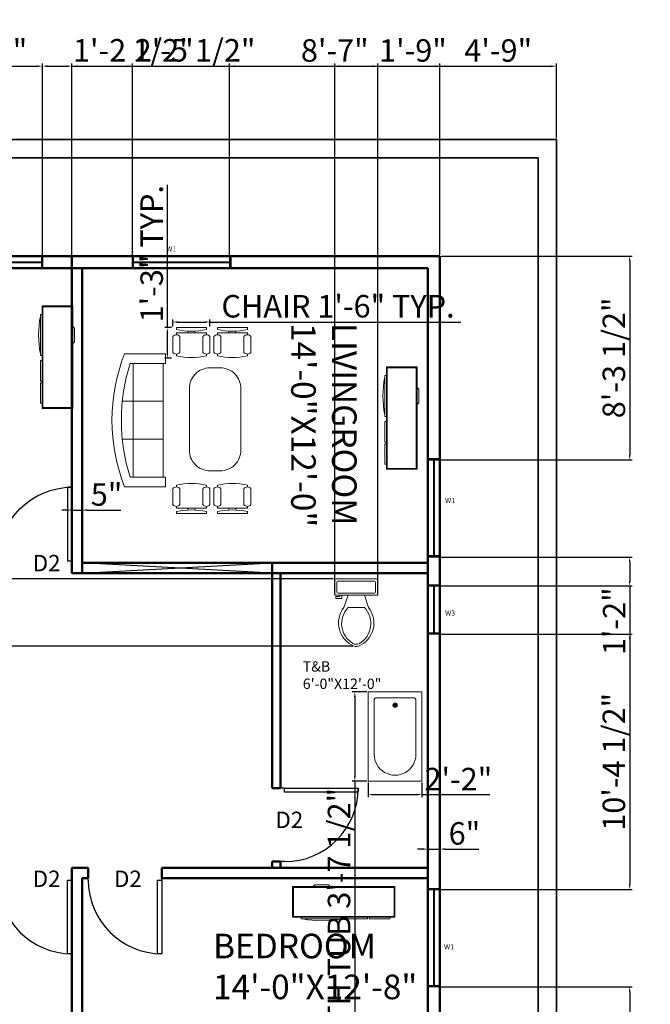
# Model space of a CAD drawing. Units: inches. Extents: x 2299 to 4423, y 1066 to 1805.
# Tile 6 of 7: x 3336 to 3645, y 1315 to 1796. Entities that reach past the tile are written whole.
import ezdxf

# ---------------------------------------------------------------- set-up
doc = ezdxf.new("R2010")
doc.units = ezdxf.units.IN
for name, color, linetype, lineweight in [('A-ANNO-DIMS', 2, 'Continuous', 18), ('A-ANNO-TEXT', 1, 'Continuous', 25), ('A-AREA-IDEN', 1, 'Continuous', 25), ('A-DOOR', 5, 'Continuous', 25), ('A-FURN', 8, 'Continuous', 18), ('A-GLAZ', 3, 'Continuous', 25), ('A-WALL', 7, 'Continuous', 50), ('C-PROP', 7, 'Continuous', 35)]:
    doc.layers.add(name, color=color, linetype=linetype, lineweight=lineweight)
doc.styles.get("Standard").update_dxf_attribs({"font": 'arial.ttf'})
doc.dimstyles.new('ISO-25', dxfattribs={"dimtxt": 11, "dimasz": 2.5, "dimexe": 1.25, "dimexo": 0.625, "dimtad": 1, "dimlunit": 4, "dimtxsty": 'Standard', "dimcen": 2.5, "dimadec": 0, "dimazin": 0, "dimtfac": 1, "dimtmove": 0, "dimatfit": 3, "dimfxl": 1, "dimarcsym": 0})

# ---------------------------------------------------------------- blocks, each defined once
blk = doc.blocks.new('*U2')
for p, q in [((0, 0), (0, -5)), ((30, 0), (30, -5))]:
    blk.add_line(p, q)
blk.add_lwpolyline([(0, 0), (0, 30), (1.75, 30), (1.75, 0)], close=True)
blk.add_arc((0, 0), 30, 0, 90)
blk = doc.blocks.new('Toilet - top')
for p, q in [((9.5, -6), (9.5, -2)), ((-10, -8.5), (-8, -8.5)), ((-10, -9.5), (-10, -8.5)), ((-7, -9.5), (-10, -9.5)), ((-8, -8.5), (-8, -8)), ((-7, -8), (-7, -9.5)), ((-4, -8), (-6, -14)), ((4, -8), (6, -14)), ((4, -14), (-4, -14))]:
    blk.add_line(p, q)
blk.add_lwpolyline([(10.5, -8), (10.5, 0), (-10.5, 0), (-10.5, -8)], close=True)
for points in [[(-9.5, -2), (-9.5, -6)], [(8.5, -1), (-8.5, -1)], [(-8.5, -7), (8.5, -7)]]:
    blk.add_lwpolyline(points)
for centre, radius, start, end in [((-8.62, -1.88), 0.884, 81.8699, 188.1301), ((8.62, -1.88), 0.884, 351.8699, 98.1301), ((-8.62, -6.12), 0.884, 171.8699, 278.1301), ((8.62, -6.12), 0.884, 261.8699, 8.1301), ((3.52, -21.58), 12.17, 141.4691, 247.9714), ((4.2, -21.82), 11.33, 136.3677, 238.9468), ((-3.52, -21.58), 12.17, 292.0284, 38.5307), ((-4.2, -21.82), 11.33, 301.053, 43.6321), ((0, -27.88), 4, 245.7318, 294.2682), ((0, -29), 4, 254.8605, 285.1395)]:
    blk.add_arc(centre, radius, start, end)
blk = doc.blocks.new('Bath Tub - 26 x 60 in.')
for p, q in [((8, -18), (10, -18)), ((9, -17), (9, -19))]:
    blk.add_line(p, q)
blk.add_lwpolyline([(0, -36), (0, 0), (60, 0), (60, -36)], close=True)
for points in [[(4, -30), (4, -6)], [(6, -4), (42, -4)], [(42, -32), (6, -32)]]:
    blk.add_lwpolyline(points)
for radius in [1.5, 1]:
    blk.add_circle((9, -18), radius)
for centre, radius, start, end in [((5.75, -5.75), 1.77, 81.8699, 188.1301), ((42, -18), 14, 270, 90), ((5.75, -30.25), 1.77, 171.8699, 278.1301)]:
    blk.add_arc(centre, radius, start, end)
blk = doc.blocks.new('Entertainment Center')
for p, q in [((-4, 0), (-5, -1)), ((4, 0), (-4, 0)), ((5, -1), (4, 0)), ((-17, -19), (-17, -1)), ((-17, -1), (43, -1)), ((-16.5, -18.5), (-16.5, -1.5)), ((-16.5, -1.5), (42.5, -1.5)), ((42.5, -1.5), (42.5, -18.5)), ((43, -1), (43, -19)), ((43, -19), (-17, -19)), ((42.5, -18.5), (-16.5, -18.5)), ((-12, -20), (-12, -19)), ((12, -20), (-12, -20)), ((12, -19), (12, -20)), ((15, -20), (15, -19)), ((27, -20), (15, -20)), ((27, -19), (27, -20)), ((28, -20), (28, -19)), ((40, -20), (28, -20)), ((40, -19), (40, -20))]:
    blk.add_line(p, q)
blk.add_arc((0, 40), 61, 259.6111, 280.3889)
blk = doc.blocks.new('Sofa - Roundback 7 ft.')
for p, q in [((-36.000027, -34), (-36.000027, -11.4696)), ((-12.00002, -32.4421), (-12.00003, -6.5971)), ((11.99997, -32.4421), (11.99998, -6.5971)), ((35.99998, -34), (35.99998, -11.4696)), ((-35.999844, -13.3819), (35.9998, -13.3819)), ((-36.000027, -32.4421), (35.99998, -32.4421))]:
    blk.add_line(p, q)
for points in [[(-36.000027, -34), (-42.000027, -34), (-42.000027, -8)], [(41.99998, -8), (41.99998, -34), (35.99998, -34)]]:
    blk.add_lwpolyline(points)
for centre, radius, start, end in [((0, -114.25), 114.25, 68.43141, 111.5686), ((-0.00001, -127.1968), 121.1968, 72.72033, 107.2797)]:
    blk.add_arc(centre, radius, start, end)
blk = doc.blocks.new('Chair - Desk')
for p, q in [((-8.5, 0), (-8.5, -1)), ((-8.5, 0), (8.5, 0)), ((8.5, 0), (8.5, -1)), ((-10.5, -5), (-10.5, -14)), ((-8.5, -3), (-8.5, -4)), ((-8.5, -3), (8.5, -3)), ((-6.5, -14), (-6.5, -5)), ((-2, -3), (-2, -1.9355)), ((2, -1.9576), (2, -3)), ((6.5, -5), (6.5, -14)), ((8.5, -3), (8.5, -4)), ((10.5, -14), (10.5, -5)), ((-8.5, -15), (-8.5, -16)), ((8.5, -15), (8.5, -16))]:
    blk.add_line(p, q)
for centre, radius, start, end in [((-8.5, -6.5), 2.5, 36.8699, 143.1301), ((0, 34.625), 36.625, 256.5803, 283.4197), ((8.5, -6.5), 2.5, 36.8699, 143.1301), ((-8.5, -12.5), 2.5, 216.8699, 323.1301), ((0, 19.625), 36.625, 256.5803, 283.4197), ((8.5, -12.5), 2.5, 216.8699, 323.1301)]:
    blk.add_arc(centre, radius, start, end)
blk = doc.blocks.new('*D26')
at = {"layer": 'A-ANNO-DIMS', "color": 0, "lineweight": -2, "transparency": 16777216}
for p, q in [((3361.75, 1589.47), (3361.75, 1555.54)), ((3366.75, 1589.47), (3366.75, 1555.54)), ((3359.25, 1556.79), (3356.75, 1556.79)), ((3361.75, 1556.79), (3366.75, 1556.79)), ((3369.25, 1556.79), (3385.64, 1556.79))]:
    blk.add_line(p, q, dxfattribs=at)
at = {"layer": 'A-ANNO-DIMS', "color": 0, "transparency": 16777216}
for points in [[(3359.25, 1557.21), (3359.25, 1556.37), (3361.75, 1556.79)], [(3369.25, 1557.21), (3369.25, 1556.37), (3366.75, 1556.79)]]:
    blk.add_solid(points, dxfattribs=at)
at = {"layer": 'Defpoints', "color": 0, "transparency": 16777216}
for p in [(3361.75, 1590.09), (3366.75, 1590.09), (3366.75, 1556.79)]:
    blk.add_point(p, dxfattribs=at)
at = {"layer": 'A-ANNO-DIMS', "color": 0, "transparency": 16777216, "insert": (3378.7, 1563.01), "char_height": 11, "attachment_point": 5}
blk.add_mtext('5"', dxfattribs=at)
blk = doc.blocks.new('*D27')
at = {"layer": 'A-ANNO-DIMS', "color": 0, "lineweight": -2, "transparency": 16777216}
for p, q in [((3535.75, 1400.25), (3535.75, 1389.83)), ((3541.75, 1400.25), (3541.75, 1389.83)), ((3533.25, 1391.08), (3530.75, 1391.08)), ((3535.75, 1391.08), (3541.75, 1391.08)), ((3544.25, 1391.08), (3560.7, 1391.08))]:
    blk.add_line(p, q, dxfattribs=at)
at = {"layer": 'A-ANNO-DIMS', "color": 0, "transparency": 16777216}
for points in [[(3533.25, 1391.5), (3533.25, 1390.66), (3535.75, 1391.08)], [(3544.25, 1391.5), (3544.25, 1390.66), (3541.75, 1391.08)]]:
    blk.add_solid(points, dxfattribs=at)
at = {"layer": 'Defpoints', "color": 0, "transparency": 16777216}
for p in [(3535.75, 1400.87), (3541.75, 1400.87), (3541.75, 1391.08)]:
    blk.add_point(p, dxfattribs=at)
at = {"layer": 'A-ANNO-DIMS', "color": 0, "transparency": 16777216, "insert": (3553.73, 1397.32), "char_height": 11, "attachment_point": 5}
blk.add_mtext('6"', dxfattribs=at)
blk = doc.blocks.new('WIN-1200')
for p, q in [((0, 0), (0, 48.07)), ((0, 48.07), (6, 48.07)), ((0, 47.57), (6, 47.57)), ((2.8, 47.57), (2.8, 0.5)), ((3.2, 47.57), (3.2, 0.5)), ((6, 48.07), (6, 0)), ((6, 0.5), (0, 0.5)), ((6, 0), (0, 0))]:
    blk.add_line(p, q)
blk = doc.blocks.new('WIN-600')
for p, q in [((0, 6), (24.07, 6)), ((0, 0), (0, 6)), ((0.5, 0), (0.5, 6)), ((23.57, 6), (23.57, 0)), ((24.07, 6), (24.07, 0)), ((24.07, 0), (0, 0)), ((0.5, 3.2), (23.57, 3.2)), ((0.5, 2.8), (23.57, 2.8))]:
    blk.add_line(p, q)
blk = doc.blocks.new('*D34')
at = {"layer": 'A-ANNO-DIMS', "color": 0, "lineweight": -2, "transparency": 16777216}
for p, q in [((3411.15, 1646.58), (3411.15, 1649.92)), ((3413.65, 1648.67), (3426.77, 1648.67)), ((3429.27, 1646.58), (3429.27, 1649.92)), ((3429.27, 1648.67), (3552.02, 1648.67))]:
    blk.add_line(p, q, dxfattribs=at)
at = {"layer": 'A-ANNO-DIMS', "color": 0, "transparency": 16777216}
for points in [[(3413.65, 1649.09), (3413.65, 1648.25), (3411.15, 1648.67)], [(3426.77, 1649.09), (3426.77, 1648.25), (3429.27, 1648.67)]]:
    blk.add_solid(points, dxfattribs=at)
at = {"layer": 'Defpoints', "color": 0, "transparency": 16777216}
for p in [(3411.15, 1645.95), (3429.27, 1648.67), (3429.27, 1645.95)]:
    blk.add_point(p, dxfattribs=at)
at = {"layer": 'A-ANNO-DIMS', "color": 0, "transparency": 16777216, "insert": (3491.9, 1654.98), "char_height": 11, "attachment_point": 5}
blk.add_mtext('CHAIR 1\'-6" TYP.', dxfattribs=at)
blk = doc.blocks.new('*D35')
at = {"layer": 'A-ANNO-DIMS', "color": 0, "lineweight": -2, "transparency": 16777216}
for p, q in [((3408.44, 1645.95), (3408.44, 1715.72)), ((3410.53, 1645.95), (3407.19, 1645.95)), ((3408.44, 1633.5), (3408.44, 1643.45)), ((3410.53, 1631), (3407.19, 1631))]:
    blk.add_line(p, q, dxfattribs=at)
at = {"layer": 'A-ANNO-DIMS', "color": 0, "transparency": 16777216}
for points in [[(3408.02, 1643.45), (3408.85, 1643.45), (3408.44, 1645.95)], [(3408.02, 1633.5), (3408.85, 1633.5), (3408.44, 1631)]]:
    blk.add_solid(points, dxfattribs=at)
at = {"layer": 'Defpoints', "color": 0, "transparency": 16777216}
for p in [(3408.44, 1645.95), (3411.15, 1645.95), (3411.15, 1631)]:
    blk.add_point(p, dxfattribs=at)
at = {"layer": 'A-ANNO-DIMS', "color": 0, "transparency": 16777216, "insert": (3402.19, 1682.08), "char_height": 11, "attachment_point": 5, "rotation": 90}
blk.add_mtext('1\'-3" TYP.', dxfattribs=at)
blk = doc.blocks.new('*D58')
at = {"layer": 'A-ANNO-DIMS', "color": 0, "lineweight": -2, "transparency": 16777216}
for p, q in [((3506.06, 1467.99), (3498.88, 1467.99)), ((3500.13, 1465.49), (3500.13, 1426.78)), ((3506.06, 1424.28), (3498.88, 1424.28)), ((3500.13, 1424.28), (3500.13, 1285.89))]:
    blk.add_line(p, q, dxfattribs=at)
at = {"layer": 'A-ANNO-DIMS', "color": 0, "transparency": 16777216}
for points in [[(3499.71, 1465.49), (3500.55, 1465.49), (3500.13, 1467.99)], [(3499.71, 1426.78), (3500.55, 1426.78), (3500.13, 1424.28)]]:
    blk.add_solid(points, dxfattribs=at)
at = {"layer": 'Defpoints', "color": 0, "transparency": 16777216}
for p in [(3506.69, 1467.99), (3500.13, 1424.28), (3506.69, 1424.28)]:
    blk.add_point(p, dxfattribs=at)
at = {"layer": 'A-ANNO-DIMS', "color": 0, "transparency": 16777216, "insert": (3493.81, 1353.83), "char_height": 11, "attachment_point": 5, "rotation": 90}
blk.add_mtext('BATH TUB 3\'-7 1/2"', dxfattribs=at)
blk = doc.blocks.new('*D59')
at = {"layer": 'A-ANNO-DIMS', "color": 0, "lineweight": -2, "transparency": 16777216}
for p, q in [((3506.69, 1423.65), (3506.69, 1416.47)), ((3532.91, 1423.65), (3532.91, 1416.47)), ((3509.19, 1417.72), (3530.41, 1417.72)), ((3532.91, 1417.72), (3566.09, 1417.72))]:
    blk.add_line(p, q, dxfattribs=at)
at = {"layer": 'A-ANNO-DIMS', "color": 0, "transparency": 16777216}
for points in [[(3509.19, 1418.14), (3509.19, 1417.31), (3506.69, 1417.72)], [(3530.41, 1418.14), (3530.41, 1417.31), (3532.91, 1417.72)]]:
    blk.add_solid(points, dxfattribs=at)
at = {"layer": 'Defpoints', "color": 0, "transparency": 16777216}
for p in [(3506.69, 1424.28), (3532.91, 1424.28), (3532.91, 1417.72)]:
    blk.add_point(p, dxfattribs=at)
at = {"layer": 'A-ANNO-DIMS', "color": 0, "transparency": 16777216, "insert": (3550.75, 1423.87), "char_height": 11, "attachment_point": 5}
blk.add_mtext('2\'-2"', dxfattribs=at)
blk = doc.blocks.new('*D60')
at = {"layer": 'A-ANNO-DIMS', "color": 0, "lineweight": -2, "transparency": 16777216}
for p, q in [((3490.3, 1515.74), (3490.3, 1775)), ((3492.8, 1773.75), (3508.8, 1773.75)), ((3511.3, 1515.74), (3511.3, 1775)), ((3511.3, 1773.75), (3543.26, 1773.75))]:
    blk.add_line(p, q, dxfattribs=at)
at = {"layer": 'A-ANNO-DIMS', "color": 0, "transparency": 16777216}
for points in [[(3492.8, 1774.16), (3492.8, 1773.33), (3490.3, 1773.75)], [(3508.8, 1774.16), (3508.8, 1773.33), (3511.3, 1773.75)]]:
    blk.add_solid(points, dxfattribs=at)
at = {"layer": 'Defpoints', "color": 0, "transparency": 16777216}
for p in [(3511.3, 1773.75), (3490.3, 1515.12), (3511.3, 1515.12)]:
    blk.add_point(p, dxfattribs=at)
at = {"layer": 'A-ANNO-DIMS', "color": 0, "transparency": 16777216, "insert": (3528.53, 1779.99), "char_height": 11, "attachment_point": 5}
blk.add_mtext('1\'-9"', dxfattribs=at)
blk = doc.blocks.new('*D61')
at = {"layer": 'A-ANNO-DIMS', "color": 0, "lineweight": -2, "transparency": 16777216}
for p, q in [((3489.68, 1523.12), (3081.7, 1523.12)), ((3082.95, 1520.62), (3082.95, 1492.76)), ((3499.13, 1490.26), (3081.7, 1490.26))]:
    blk.add_line(p, q, dxfattribs=at)
at = {"layer": 'A-ANNO-DIMS', "color": 0, "transparency": 16777216}
for points in [[(3082.53, 1520.62), (3083.37, 1520.62), (3082.95, 1523.12)], [(3082.53, 1492.76), (3083.37, 1492.76), (3082.95, 1490.26)]]:
    blk.add_solid(points, dxfattribs=at)
at = {"layer": 'Defpoints', "color": 0, "transparency": 16777216}
for p in [(3490.3, 1523.12), (3082.95, 1490.26), (3499.76, 1490.26)]:
    blk.add_point(p, dxfattribs=at)
at = {"layer": 'A-ANNO-DIMS', "color": 0, "transparency": 16777216, "insert": (3076.71, 1506.69), "char_height": 11, "attachment_point": 5, "rotation": 90}
blk.add_mtext('2\'-9"', dxfattribs=at)
blk = doc.blocks.new('*D93')
at = {"layer": 'A-ANNO-DIMS', "color": 0, "lineweight": -2, "transparency": 16777216}
for p, q in [((3299.28, 1681.57), (3299.28, 1775)), ((3301.78, 1773.75), (3344.85, 1773.75)), ((3347.35, 1681.57), (3347.35, 1775))]:
    blk.add_line(p, q, dxfattribs=at)
at = {"layer": 'A-ANNO-DIMS', "color": 0, "transparency": 16777216}
for points in [[(3301.78, 1774.16), (3301.78, 1773.33), (3299.28, 1773.75)], [(3344.85, 1774.16), (3344.85, 1773.33), (3347.35, 1773.75)]]:
    blk.add_solid(points, dxfattribs=at)
at = {"layer": 'Defpoints', "color": 0, "transparency": 16777216}
for p in [(3347.35, 1773.75), (3299.28, 1680.95), (3347.35, 1680.95)]:
    blk.add_point(p, dxfattribs=at)
at = {"layer": 'A-ANNO-DIMS', "color": 0, "transparency": 16777216, "insert": (3323.32, 1779.99), "char_height": 11, "attachment_point": 5}
blk.add_mtext('4\'-0"', dxfattribs=at)
blk = doc.blocks.new('*D94')
at = {"layer": 'A-ANNO-DIMS', "color": 0, "lineweight": -2, "transparency": 16777216}
for p, q in [((3347.35, 1681.57), (3347.35, 1775)), ((3349.85, 1773.75), (3359.25, 1773.75)), ((3361.75, 1681.57), (3361.75, 1775)), ((3361.75, 1773.75), (3419.34, 1773.75))]:
    blk.add_line(p, q, dxfattribs=at)
at = {"layer": 'A-ANNO-DIMS', "color": 0, "transparency": 16777216}
for points in [[(3349.85, 1774.16), (3349.85, 1773.33), (3347.35, 1773.75)], [(3359.25, 1774.16), (3359.25, 1773.33), (3361.75, 1773.75)]]:
    blk.add_solid(points, dxfattribs=at)
at = {"layer": 'Defpoints', "color": 0, "transparency": 16777216}
for p in [(3361.75, 1773.75), (3347.35, 1680.95), (3361.75, 1680.95)]:
    blk.add_point(p, dxfattribs=at)
at = {"layer": 'A-ANNO-DIMS', "color": 0, "transparency": 16777216, "insert": (3391.79, 1780.06), "char_height": 11, "attachment_point": 5}
blk.add_mtext('1\'-2 1/2"', dxfattribs=at)
blk = doc.blocks.new('*D95')
at = {"layer": 'A-ANNO-DIMS', "color": 0, "lineweight": -2, "transparency": 16777216}
for p, q in [((3361.75, 1681.57), (3361.75, 1775)), ((3364.25, 1773.75), (3388.83, 1773.75)), ((3391.33, 1681.57), (3391.33, 1775)), ((3391.33, 1773.75), (3450.14, 1773.75))]:
    blk.add_line(p, q, dxfattribs=at)
at = {"layer": 'A-ANNO-DIMS', "color": 0, "transparency": 16777216}
for points in [[(3364.25, 1774.16), (3364.25, 1773.33), (3361.75, 1773.75)], [(3388.83, 1774.16), (3388.83, 1773.33), (3391.33, 1773.75)]]:
    blk.add_solid(points, dxfattribs=at)
at = {"layer": 'Defpoints', "color": 0, "transparency": 16777216}
for p in [(3391.33, 1773.75), (3361.75, 1680.95), (3391.33, 1680.95)]:
    blk.add_point(p, dxfattribs=at)
at = {"layer": 'A-ANNO-DIMS', "color": 0, "transparency": 16777216, "insert": (3421.98, 1780.06), "char_height": 11, "attachment_point": 5}
blk.add_mtext('2\'-5 1/2"', dxfattribs=at)
blk = doc.blocks.new('*D96')
at = {"layer": 'A-ANNO-DIMS', "color": 0, "lineweight": -2, "transparency": 16777216}
for p, q in [((3438.9, 1681.57), (3438.9, 1775)), ((3441.4, 1773.75), (3539.25, 1773.75)), ((3541.75, 1681.57), (3541.75, 1775))]:
    blk.add_line(p, q, dxfattribs=at)
at = {"layer": 'A-ANNO-DIMS', "color": 0, "transparency": 16777216}
for points in [[(3441.4, 1774.16), (3441.4, 1773.33), (3438.9, 1773.75)], [(3539.25, 1774.16), (3539.25, 1773.33), (3541.75, 1773.75)]]:
    blk.add_solid(points, dxfattribs=at)
at = {"layer": 'Defpoints', "color": 0, "transparency": 16777216}
for p in [(3541.75, 1773.75), (3438.9, 1680.95), (3541.75, 1680.95)]:
    blk.add_point(p, dxfattribs=at)
at = {"layer": 'A-ANNO-DIMS', "color": 0, "transparency": 16777216, "insert": (3490.32, 1779.99), "char_height": 11, "attachment_point": 5}
blk.add_mtext('8\'-7"', dxfattribs=at)
blk = doc.blocks.new('*D97')
at = {"layer": 'A-ANNO-DIMS', "color": 0, "lineweight": -2, "transparency": 16777216}
for p, q in [((3541.75, 1681.57), (3541.75, 1775)), ((3544.25, 1773.75), (3596.25, 1773.75)), ((3598.75, 1738.57), (3598.75, 1775))]:
    blk.add_line(p, q, dxfattribs=at)
at = {"layer": 'A-ANNO-DIMS', "color": 0, "transparency": 16777216}
for points in [[(3544.25, 1774.16), (3544.25, 1773.33), (3541.75, 1773.75)], [(3596.25, 1774.16), (3596.25, 1773.33), (3598.75, 1773.75)]]:
    blk.add_solid(points, dxfattribs=at)
at = {"layer": 'Defpoints', "color": 0, "transparency": 16777216}
for p in [(3598.75, 1773.75), (3598.75, 1737.95), (3541.75, 1680.95)]:
    blk.add_point(p, dxfattribs=at)
at = {"layer": 'A-ANNO-DIMS', "color": 0, "transparency": 16777216, "insert": (3570.25, 1779.99), "char_height": 11, "attachment_point": 5}
blk.add_mtext('4\'-9"', dxfattribs=at)
blk = doc.blocks.new('*D105')
at = {"layer": 'A-ANNO-DIMS', "color": 0, "lineweight": -2, "transparency": 16777216}
for p, q in [((3542.37, 1680.95), (3635.8, 1680.95)), ((3634.55, 1678.45), (3634.55, 1583.91)), ((3542.37, 1581.41), (3635.8, 1581.41))]:
    blk.add_line(p, q, dxfattribs=at)
at = {"layer": 'A-ANNO-DIMS', "color": 0, "transparency": 16777216}
for points in [[(3634.13, 1678.45), (3634.97, 1678.45), (3634.55, 1680.95)], [(3634.13, 1583.91), (3634.97, 1583.91), (3634.55, 1581.41)]]:
    blk.add_solid(points, dxfattribs=at)
at = {"layer": 'Defpoints', "color": 0, "transparency": 16777216}
for p in [(3541.75, 1680.95), (3541.75, 1581.41), (3634.55, 1581.41)]:
    blk.add_point(p, dxfattribs=at)
at = {"layer": 'A-ANNO-DIMS', "color": 0, "transparency": 16777216, "insert": (3628.23, 1631.18), "char_height": 11, "attachment_point": 5, "rotation": 90}
blk.add_mtext('8\'-3 1/2"', dxfattribs=at)
blk = doc.blocks.new('*D106')
at = {"layer": 'A-ANNO-DIMS', "color": 0, "lineweight": -2, "transparency": 16777216}
for p, q in [((3542.37, 1533.84), (3635.8, 1533.84)), ((3634.55, 1531.34), (3634.55, 1522.18)), ((3542.37, 1519.68), (3635.8, 1519.68)), ((3634.55, 1519.68), (3634.55, 1487.72))]:
    blk.add_line(p, q, dxfattribs=at)
at = {"layer": 'A-ANNO-DIMS', "color": 0, "transparency": 16777216}
for points in [[(3634.13, 1531.34), (3634.97, 1531.34), (3634.55, 1533.84)], [(3634.13, 1522.18), (3634.97, 1522.18), (3634.55, 1519.68)]]:
    blk.add_solid(points, dxfattribs=at)
at = {"layer": 'Defpoints', "color": 0, "transparency": 16777216}
for p in [(3541.75, 1533.84), (3541.75, 1519.68), (3634.55, 1519.68)]:
    blk.add_point(p, dxfattribs=at)
at = {"layer": 'A-ANNO-DIMS', "color": 0, "transparency": 16777216, "insert": (3628.4, 1502.45), "char_height": 11, "attachment_point": 5, "rotation": 90}
blk.add_mtext('1\'-2"', dxfattribs=at)
blk = doc.blocks.new('*D107')
at = {"layer": 'A-ANNO-DIMS', "color": 0, "lineweight": -2, "transparency": 16777216}
for p, q in [((3542.37, 1496.11), (3635.8, 1496.11)), ((3634.55, 1493.61), (3634.55, 1373.86)), ((3542.37, 1371.36), (3635.8, 1371.36))]:
    blk.add_line(p, q, dxfattribs=at)
at = {"layer": 'A-ANNO-DIMS', "color": 0, "transparency": 16777216}
for points in [[(3634.13, 1493.61), (3634.97, 1493.61), (3634.55, 1496.11)], [(3634.13, 1373.86), (3634.97, 1373.86), (3634.55, 1371.36)]]:
    blk.add_solid(points, dxfattribs=at)
at = {"layer": 'Defpoints', "color": 0, "transparency": 16777216}
for p in [(3541.75, 1496.11), (3541.75, 1371.36), (3634.55, 1371.36)]:
    blk.add_point(p, dxfattribs=at)
at = {"layer": 'A-ANNO-DIMS', "color": 0, "transparency": 16777216, "insert": (3628.24, 1433.74), "char_height": 11, "attachment_point": 5, "rotation": 90}
blk.add_mtext('10\'-4 1/2"', dxfattribs=at)
blk = doc.blocks.new('*D108')
at = {"layer": 'A-ANNO-DIMS', "color": 0, "lineweight": -2, "transparency": 16777216}
for p, q in [((3542.37, 1323.79), (3635.8, 1323.79)), ((3634.55, 1321.29), (3634.55, 1221.45)), ((3542.37, 1218.95), (3635.8, 1218.95))]:
    blk.add_line(p, q, dxfattribs=at)
at = {"layer": 'A-ANNO-DIMS', "color": 0, "transparency": 16777216}
for points in [[(3634.13, 1321.29), (3634.97, 1321.29), (3634.55, 1323.79)], [(3634.13, 1221.45), (3634.97, 1221.45), (3634.55, 1218.95)]]:
    blk.add_solid(points, dxfattribs=at)
at = {"layer": 'Defpoints', "color": 0, "transparency": 16777216}
for p in [(3541.75, 1323.79), (3541.75, 1218.95), (3634.55, 1218.95)]:
    blk.add_point(p, dxfattribs=at)
at = {"layer": 'A-ANNO-DIMS', "color": 0, "transparency": 16777216, "insert": (3628.31, 1271.37), "char_height": 11, "attachment_point": 5, "rotation": 90}
blk.add_mtext('8\'-9"', dxfattribs=at)

msp = doc.modelspace()

# ---------------------------------------------------------------- linework, layer by layer
at = {"layer": 'A-FURN'}
msp.add_lwpolyline([(3419.211, 1616.233, -0.4142136), (3429.281, 1626.303), (3434.316, 1626.303, -0.4142136), (3444.386, 1616.233), (3444.386, 1586.023, -0.4142136), (3434.316, 1575.953), (3429.281, 1575.953, -0.4142136), (3419.211, 1586.023)], format="xyb", close=True, dxfattribs=at)
at = {"layer": 'A-GLAZ'}
for p, q in [((3366.749, 1525.945), (3459.749, 1530.945)), ((3459.749, 1525.945), (3366.749, 1530.945))]:
    msp.add_line(p, q, dxfattribs=at)
at = {"layer": 'A-WALL'}
for p, q in [((3175.749, 1680.945), (3541.749, 1680.945)), ((3361.749, 1530.945), (3361.749, 1680.945)), ((3541.749, 1680.945), (3541.749, 1429.945)), ((3181.749, 1674.945), (3535.749, 1674.945)), ((3366.749, 1530.945), (3366.749, 1674.945)), ((3395.749, 1674.945), (3535.749, 1674.945)), ((3535.749, 1674.945), (3535.749, 1477.945)), ((3361.749, 1525.945), (3361.749, 1530.945)), ((3366.749, 1530.945), (3535.749, 1530.945)), ((3366.749, 1530.945), (3366.749, 1525.945)), ((3459.749, 1530.945), (3459.749, 1429.945)), ((3366.749, 1525.945), (3361.749, 1525.945)), ((3366.749, 1525.945), (3535.749, 1525.945)), ((3463.749, 1525.945), (3463.749, 1429.945)), ((3535.749, 1525.945), (3535.749, 1429.945)), ((3459.749, 1429.945), (3459.749, 1420.945)), ((3463.749, 1429.945), (3463.749, 1420.945)), ((3535.749, 1429.945), (3535.749, 1349.945)), ((3541.749, 1429.945), (3541.749, 1344.945)), ((3459.749, 1420.945), (3463.749, 1420.945)), ((3361.749, 1224.945), (3361.749, 1381.945)), ((3369.749, 1381.945), (3361.749, 1381.945)), ((3369.749, 1376.945), (3369.749, 1381.945)), ((3535.749, 1381.945), (3405.749, 1381.945)), ((3405.749, 1381.945), (3405.749, 1376.945)), ((3463.749, 1384.945), (3459.749, 1384.945)), ((3459.749, 1384.945), (3459.749, 1381.945)), ((3463.749, 1381.945), (3463.749, 1384.945)), ((3463.749, 1384.945), (3463.749, 1381.945)), ((3366.749, 1224.945), (3366.749, 1376.945)), ((3366.749, 1376.945), (3369.749, 1376.945)), ((3369.749, 1376.945), (3366.749, 1376.945)), ((3535.749, 1376.945), (3405.749, 1376.945)), ((3535.749, 1224.945), (3535.749, 1349.945)), ((3541.749, 1218.945), (3541.749, 1344.945))]:
    msp.add_line(p, q, dxfattribs=at)
at = {"layer": 'C-PROP'}
for p, q in [((3118.749, 1737.945), (3598.749, 1737.945)), ((3598.749, 1737.945), (3598.749, 1161.945)), ((3127.749, 1728.945), (3589.749, 1728.945)), ((3589.749, 1728.945), (3589.749, 1170.945))]:
    msp.add_line(p, q, dxfattribs=at)

# ---------------------------------------------------------------- block references
at = {"layer": 'A-DOOR', "xscale": -1.199999999999999, "yscale": 1.199999999999999, "zscale": 1.199999999999999}
msp.add_blockref('*U2', (3361.749, 1531.945), dxfattribs=at)
at = {"layer": 'A-DOOR', "xscale": 1.199999999999999, "yscale": 1.199999999999999, "zscale": 1.199999999999999}
for p, rotation in [((3465.749, 1420.945), 270), ((3361.749, 1375.945), 180), ((3405.749, 1375.945), 180)]:
    msp.add_blockref('*U2', p, dxfattribs=dict(at, rotation=rotation))
at = {"layer": 'A-FURN'}
for name, p, xscale, yscale, zscale, rotation in [('Entertainment Center', (3363, 1642.362), 0.8342103315264846, 0.8342103315264846, 0.8342103315264846, 270), ('Sofa - Roundback 7 ft.', (3381.316, 1600.667), 0.7724308018975573, 0.7724308018975573, 0.7724308018975573, 90), ('Entertainment Center', (3531.412, 1612.569), 0.8342103315264846, 0.8342103315264846, 0.8342103315264846, 270), ('Chair - Desk', (3420.212, 1555.148), -0.8626440446238717, 0.8626440446238717, 0.8626440446238717, 180), ('Chair - Desk', (3440.269, 1555.148), -0.8626440446238717, 0.8626440446238717, 0.8626440446238717, 180), ('Bath Tub - 26 x 60 in.', (3532.914, 1467.993), 0.7285583953973916, 0.7285583953973916, 0.7285583953973916, 270)]:
    msp.add_blockref(name, p, dxfattribs=dict(at, xscale=xscale, yscale=yscale, zscale=zscale, rotation=rotation))
for name, p, xscale, yscale, zscale in [('Chair - Desk', (3420.212, 1645.952), 0.8626440446238717, 0.8626440446238717, 0.8626440446238717), ('Chair - Desk', (3440.269, 1645.952), 0.8626440446238717, 0.8626440446238717, 0.8626440446238717), ('Entertainment Center', (3483.857, 1373.618), 0.8342103315264846, 0.8342103315264846, 0.8342103315264846)]:
    msp.add_blockref(name, p, dxfattribs=dict(at, xscale=xscale, yscale=yscale, zscale=zscale))
msp.add_blockref('Toilet - top', (3500.802, 1523.118), dxfattribs=at)
at = {"layer": 'A-GLAZ'}
for name, p, rotation in [('WIN-1200', (3347.352, 1674.945), 90.00000000000188), ('WIN-1200', (3439.4, 1674.945), 90.00000000000014), ('WIN-600', (3535.749, 1520.18), 270.0000000000036)]:
    msp.add_blockref(name, p, dxfattribs=dict(at, rotation=rotation))
for p in [(3535.749, 1533.842), (3535.749, 1323.793)]:
    msp.add_blockref('WIN-1200', p, dxfattribs=at)

# ---------------------------------------------------------------- texts
at = {"layer": 'A-ANNO-TEXT', "char_height": 2.5, "attachment_point": 1}
for s, insert in [('W1', (3407.904, 1685.701)), ('W1', (3544.254, 1562.68)), ('W3', (3544.254, 1507.716)), ('W1', (3543.739, 1344.547))]:
    msp.add_mtext(s, dxfattribs=dict(at, insert=insert))
at = {"layer": 'A-ANNO-TEXT', "char_height": 8, "attachment_point": 1}
for insert in [(3342.61, 1534.88), (3461.299, 1409.367), (3342.61, 1380.579), (3382.365, 1380.579)]:
    msp.add_mtext_dynamic_manual_height_columns('D2', width=1.11117, gutter_width=12.5, heights=[0], dxfattribs=dict(at, insert=insert))
at = {"layer": 'A-AREA-IDEN', "insert": (3500.99, 1648.264), "char_height": 12, "attachment_point": 1, "rotation": 270}
msp.add_mtext_dynamic_manual_height_columns('LIVINGROOM\\P14\'-0"X12\'-0"', width=9.28623, gutter_width=12.5, heights=[0], dxfattribs=at)
at = {"layer": 'A-AREA-IDEN', "attachment_point": 1}
for s, width, gutter_width, insert, char_height in [('T&B\\P6\'-0"X12\'-0"', 2.46662, 25.4, (3474.661, 1482.891), 5.07992), ('BEDROOM\\P14\'-0"X12\'-8"', 9.28623, 12.5, (3430.771, 1349.725), 12)]:
    msp.add_mtext_dynamic_manual_height_columns(s, width=width, gutter_width=gutter_width, heights=[0], dxfattribs=dict(at, insert=insert, char_height=char_height))

# ---------------------------------------------------------------- dimensions: what is measured, and where the dimension line sits
at = {"layer": 'A-ANNO-DIMS'}
for base, p1, p2, override, picture, middle in [((3361.749, 1773.745), (3347.352, 1680.945), (3361.749, 1680.945), {"dimdec": 1, "dimlfac": 1, "dimrnd": 0, "dimzin": 1, "dimdsep": 46, "dimlunit": 4, "dimfrac": 2}, '*D94', (3391.793, 1780.058)), ((3391.329, 1773.745), (3361.749, 1680.945), (3391.329, 1680.945), {"dimdec": 1, "dimlfac": 1, "dimrnd": 0, "dimzin": 1, "dimdsep": 46, "dimlunit": 4, "dimfrac": 2}, '*D95', (3421.984, 1780.058)), ((3347.352, 1773.745), (3299.282, 1680.945), (3347.352, 1680.945), {"dimdec": 1, "dimlfac": 1, "dimrnd": 0, "dimzin": 1, "dimdsep": 46, "dimlunit": 4, "dimfrac": 2}, '*D93', (3323.317, 1779.987)), ((3541.749, 1773.745), (3438.9, 1680.945), (3541.749, 1680.945), {"dimdec": 1, "dimlfac": 1, "dimrnd": 0, "dimzin": 1, "dimdsep": 46, "dimlunit": 4, "dimfrac": 2}, '*D96', (3490.325, 1779.987)), ((3511.302, 1773.745), (3490.302, 1515.118), (3511.302, 1515.118), {"dimdec": 1, "dimlfac": 1, "dimrnd": 0, "dimzin": 1, "dimdsep": 46, "dimlunit": 4, "dimfrac": 2}, '*D60', (3528.529, 1779.987)), ((3598.749, 1773.745), (3541.749, 1680.945), (3598.749, 1737.945), {"dimdec": 1, "dimlfac": 1, "dimrnd": 0, "dimzin": 1, "dimdsep": 46, "dimlunit": 4, "dimfrac": 2}, '*D97', (3570.249, 1779.987)), ((3366.749, 1556.789), (3361.749, 1590.094), (3366.749, 1590.094), {"dimclrd": 0, "dimclre": 0, "dimclrt": 0}, '*D26', (3378.696, 1563.008)), ((3532.914, 1417.723), (3506.686, 1424.28), (3532.914, 1424.28), {"dimdec": 1, "dimrnd": 0, "dimzin": 1, "dimlunit": 4, "dimfrac": 2}, '*D59', (3550.753, 1423.87)), ((3541.749, 1391.078), (3535.749, 1400.872), (3541.749, 1400.872), {"dimclrd": 0, "dimclre": 0, "dimclrt": 0}, '*D27', (3553.726, 1397.32))]:
    dim = msp.add_linear_dim(base=base, p1=p1, p2=p2, dimstyle='ISO-25', override=override, dxfattribs=at)
    dim.commit()
    dim.dimension.update_dxf_attribs({"geometry": picture, "text_midpoint": middle})
for base, p1, p2, angle, text, picture, middle in [((3408.437, 1645.952), (3411.154, 1631), (3411.154, 1645.952), 90, '<> TYP.', '*D35', (3402.192, 1682.085)), ((3500.129, 1424.28), (3506.686, 1467.993), (3506.686, 1424.28), 270, 'BATH TUB <>', '*D58', (3493.812, 1353.834))]:
    dim = msp.add_linear_dim(base=base, p1=p1, p2=p2, angle=angle, text=text, dimstyle='ISO-25', override={"dimdec": 1, "dimrnd": 0, "dimzin": 1, "dimlunit": 4, "dimfrac": 2}, dxfattribs=at)
    dim.commit()
    dim.dimension.update_dxf_attribs({"geometry": picture, "text_midpoint": middle})
dim = msp.add_linear_dim(base=(3429.27, 1648.67), p1=(3411.154, 1645.952), p2=(3429.27, 1645.952), text='CHAIR <> TYP.', dimstyle='ISO-25', override={"dimdec": 1, "dimrnd": 0, "dimzin": 1, "dimlunit": 4, "dimfrac": 2}, dxfattribs=at)
dim.commit()
dim.dimension.update_dxf_attribs({"geometry": '*D34', "text_midpoint": (3491.897, 1654.982)})
for base, p1, p2, picture, middle in [((3634.549, 1581.413), (3541.749, 1680.945), (3541.749, 1581.413), '*D105', (3628.233, 1631.179)), ((3634.549, 1519.68), (3541.749, 1533.842), (3541.749, 1519.68), '*D106', (3628.402, 1502.452)), ((3082.949, 1490.257), (3490.302, 1523.118), (3499.757, 1490.257), '*D61', (3076.708, 1506.687)), ((3634.549, 1371.364), (3541.749, 1496.109), (3541.749, 1371.364), '*D107', (3628.237, 1433.737)), ((3634.549, 1218.945), (3541.749, 1323.793), (3541.749, 1218.945), '*D108', (3628.308, 1271.369))]:
    dim = msp.add_linear_dim(base=base, p1=p1, p2=p2, angle=90, dimstyle='ISO-25', override={"dimdec": 1, "dimlfac": 1, "dimrnd": 0, "dimzin": 1, "dimdsep": 46, "dimlunit": 4, "dimfrac": 2}, dxfattribs=at)
    dim.commit()
    dim.dimension.update_dxf_attribs({"geometry": picture, "text_midpoint": middle})

doc.saveas('drawing.dxf')
